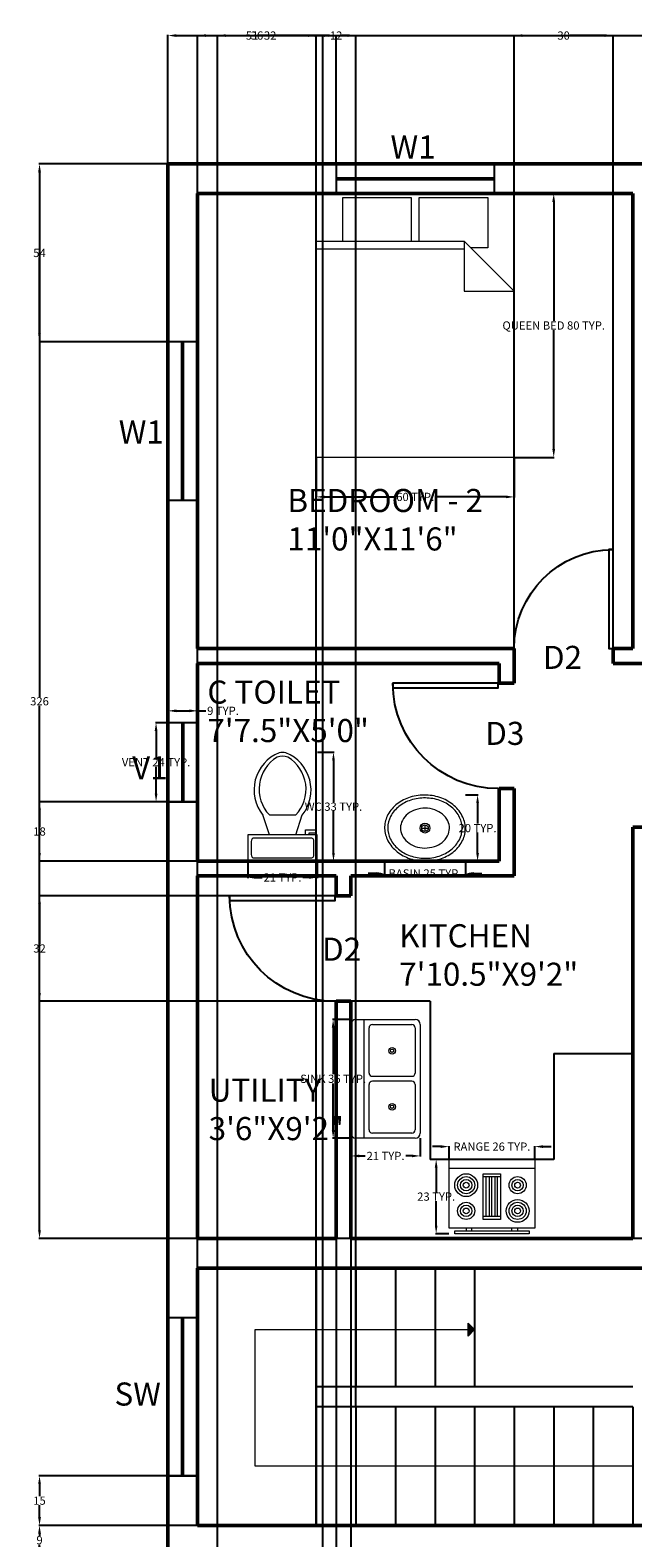
# Model space of a CAD drawing. Units: inches. Extents: x 227 to 711, y 218 to 1048.
# Tile 4 of 5: x 227 to 410, y 590 to 1048. Entities that reach past the tile are written whole.
import ezdxf

# ---------------------------------------------------------------- set-up
doc = ezdxf.new("R2010")
doc.units = ezdxf.units.IN
doc.header["$MEASUREMENT"] = 0
for name, color, linetype, lineweight in [('A-ANNO-DIMS', 2, 'Continuous', 18), ('A-ANNO-SYMB', 85, 'Continuous', 18), ('A-ANNO-TEXT', 70, 'Continuous', 18), ('A-AREA-IDEN', 70, 'Continuous', 25), ('A-FLOR-CASE', 32, 'Continuous', 25), ('A-FLOR-FIXT', 140, 'Continuous', 18), ('A-FURN', 8, 'Continuous', 18), ('A-WALL', 10, 'Continuous', 50), ('DOORS', 30, 'Continuous', 25), ('EQUIPMENTS', 140, 'Continuous', 18), ('STAIRCASE', 220, 'Continuous', 25), ('WINDOWS', 50, 'Continuous', 25)]:
    doc.layers.add(name, color=color, linetype=linetype, lineweight=lineweight)
doc.styles.get("Standard").update_dxf_attribs({"font": 'arial.ttf'})
doc.dimstyles.get("Standard").update_dxf_attribs({"dimtxt": 2.5, "dimasz": 2.5, "dimexe": 0.18, "dimexo": 0.0625, "dimgap": 0.09, "dimtad": 0, "dimtih": 1, "dimtoh": 1, "dimzin": 0, "dimdsep": 46, "dimlunit": 3, "dimtxsty": 'Standard', "dimcen": 0.09, "dimadec": 0, "dimazin": 0, "dimtfac": 1, "dimtofl": 0, "dimtmove": 0, "dimatfit": 3, "dimfxl": 1, "dimtolj": 1, "dimtzin": 0, "dimarcsym": 0})

# ---------------------------------------------------------------- blocks, each defined once
blk = doc.blocks.new('*U2')
for p, q in [((0, 0), (0, -6)), ((40, 0), (40, -6))]:
    blk.add_line(p, q)
blk.add_lwpolyline([(0, 0), (0, 40), (1.75, 40), (1.75, 0)], close=True)
blk.add_arc((0, 0), 40, 0, 90)
blk = doc.blocks.new('Bed - Queen')
for p, q in [((0, -80.00003), (0, 0)), ((0, 0), (59.99999, 0)), ((59.99999, 0), (59.99999, -80.00003)), ((7.99999, -1.2), (28.79998, -1.2)), ((7.99999, -14.4), (7.99999, -1.2)), ((28.79998, -1.2), (28.79998, -14.4)), ((31.19999, -1.2), (51.99999, -1.2)), ((31.19999, -14.4), (31.19999, -1.2)), ((51.99999, -1.2), (51.99999, -16.4)), ((0, -14.4), (44.8, -14.4)), ((44.8, -16.8), (0, -16.8)), ((59.99999, -29.6), (44.8, -14.4)), ((44.8, -14.4), (44.8, -29.6)), ((51.99999, -16.4), (46.79936, -16.4)), ((44.8, -29.6), (59.99999, -29.6)), ((59.99999, -80.00003), (0, -80.00003))]:
    blk.add_line(p, q)
blk = doc.blocks.new('Toilet - top')
for p, q in [((9.5, -6), (9.5, -2)), ((-10, -8.5), (-8, -8.5)), ((-10, -9.5), (-10, -8.5)), ((-8, -8.5), (-8, -8)), ((-7, -8), (-7, -9.5)), ((-4, -8), (-6, -14)), ((4, -8), (6, -14)), ((-7, -9.5), (-10, -9.5)), ((4, -14), (-4, -14))]:
    blk.add_line(p, q)
blk.add_lwpolyline([(10.5, -8), (10.5, 0), (-10.5, 0), (-10.5, -8)], close=True)
for points in [[(-9.5, -2), (-9.5, -6)], [(8.5, -1), (-8.5, -1)], [(-8.5, -7), (8.5, -7)]]:
    blk.add_lwpolyline(points)
for centre, radius, start, end in [((-8.62, -1.88), 0.884, 81.8699, 188.1301), ((8.62, -1.88), 0.884, 351.8699, 98.1301), ((-8.62, -6.12), 0.884, 171.8699, 278.1301), ((8.62, -6.12), 0.884, 261.8699, 8.1301), ((3.52, -21.58), 12.17, 141.4691, 247.9714), ((4.2, -21.82), 11.33, 136.3677, 238.9468), ((-3.52, -21.58), 12.17, 292.0284, 38.5307), ((-4.2, -21.82), 11.33, 301.053, 43.6321), ((0, -27.88), 4, 245.7318, 294.2682), ((0, -29), 4, 254.8605, 285.1395)]:
    blk.add_arc(centre, radius, start, end)
blk = doc.blocks.new('Sink - Oval top')
for p, q in [((-1, 0), (1, 0)), ((0, 1), (0, -1))]:
    blk.add_line(p, q)
for points in [[(-12.23, 0.39, 0.117634), (-11.46, -3.36, 0.104469), (-8.88, -6.8, 0.090016), (-5.08, -9.07, 0.08192), (-0.32, -10.02, 0.08192), (4.49, -9.38, 0.090016), (8.42, -7.36, 0.104469), (11.22, -4.09, 0.117634), (12.23, -0.39, 0.117634), (11.46, 3.36, 0.104469), (8.88, 6.8, 0.090016), (5.08, 9.07, 0.08192), (0.32, 10.02, 0.08192), (-4.49, 9.38, 0.090016), (-8.42, 7.36, 0.104469), (-11.22, 4.09, 0.117634)], [(-11.29, 0.16, 0.118622), (-10.52, -3.25, 0.104678), (-8.07, -6.36, 0.089562), (-4.54, -8.37, 0.081185), (-0.13, -9.15, 0.081185), (4.3, -8.49, 0.089562), (7.89, -6.58, 0.104678), (10.42, -3.55, 0.118622), (11.29, -0.16, 0.118622), (10.52, 3.25, 0.104678), (8.07, 6.36, 0.089562), (4.54, 8.37, 0.081185), (0.13, 9.15, 0.081185), (-4.3, 8.49, 0.089562), (-7.89, 6.58, 0.104678), (-10.42, 3.55, 0.118622)], [(-7.42, 0.08, 0.118283), (-6.91, -2.17, 0.104607), (-5.29, -4.21, 0.089718), (-2.97, -5.53, 0.081436), (-0.07, -6.04, 0.081436), (2.84, -5.59, 0.089718), (5.2, -4.33, 0.104607), (6.86, -2.32, 0.118283), (7.42, -0.08, 0.118283), (6.91, 2.17, 0.104607), (5.29, 4.21, 0.089718), (2.97, 5.53, 0.081436), (0.07, 6.04, 0.081436), (-2.84, 5.59, 0.089718), (-5.2, 4.33, 0.104607), (-6.86, 2.32, 0.118283)]]:
    blk.add_lwpolyline(points, format="xyb", close=True)
for radius in [1.5, 1]:
    blk.add_circle((0, 0), radius)
blk = doc.blocks.new('Range-Oven - 30 in top')
for p, q in [((0, -3), (30, -3)), ((12, -6), (18, -6)), ((13, -20), (13, -6)), ((14, -6), (14, -20)), ((15, -20), (15, -6)), ((16, -6), (16, -20)), ((17, -20), (17, -6)), ((18, -20), (12, -20)), ((6, -24), (6, -25)), ((8, -25), (8, -24)), ((22, -25), (22, -24)), ((24, -24), (24, -25))]:
    blk.add_line(p, q)
for points in [[(0, -24), (0, 0), (30, 0), (30, -24)], [(12, -21), (12, -5), (18, -5), (18, -21)], [(2, -26), (2, -25), (28, -25), (28, -26)]]:
    blk.add_lwpolyline(points, close=True)
for centre, radius in [((6, -9), 4), ((6, -9), 3), ((6, -9), 2), ((6, -9), 1), ((24, -9), 3), ((24, -9), 2), ((24, -9), 1), ((6, -18), 3), ((24, -18), 4), ((24, -18), 3), ((6, -18), 2), ((6, -18), 1), ((24, -18), 2), ((24, -18), 1)]:
    blk.add_circle(centre, radius)
blk = doc.blocks.new('Sink-double - 36 in top')
for p, q in [((-18, -4), (18, -4)), ((-0.75, -18.5), (-0.75, -6.5)), ((0.75, -6.5), (0.75, -18.5))]:
    blk.add_line(p, q)
for points in [[(-16.5, 0), (16.5, 0)], [(-18, -19.5), (-18, -1.5)], [(18, -1.5), (18, -19.5)], [(-16.5, -18.5), (-16.5, -6.5)], [(-15.5, -5.5), (-1.75, -5.5)], [(1.75, -5.5), (15.5, -5.5)], [(16.5, -6.5), (16.5, -18.5)], [(16.5, -21), (-16.5, -21)], [(-1.75, -19.5), (-15.5, -19.5)], [(15.5, -19.5), (1.75, -19.5)]]:
    blk.add_lwpolyline(points)
for centre, radius in [((-8.5, -12.5), 1), ((-8.5, -12.5), 0.5), ((8.5, -12.5), 1), ((8.5, -12.5), 0.5)]:
    blk.add_circle(centre, radius)
for centre, radius, start, end in [((-16.5, -1.5), 1.5, 90, 180), ((16.5, -1.5), 1.5, 0, 90), ((-15.5, -6.5), 1, 90, 180), ((-1.75, -6.5), 1, 0, 90), ((1.75, -6.5), 1, 90, 180), ((15.5, -6.5), 1, 0, 90), ((-16.5, -19.5), 1.5, 180, 270), ((-15.5, -18.5), 1, 180, 270), ((-1.75, -18.5), 1, 270, 0), ((1.75, -18.5), 1, 180, 270), ((15.5, -18.5), 1, 270, 0), ((16.5, -19.5), 1.5, 270, 0)]:
    blk.add_arc(centre, radius, start, end)
blk = doc.blocks.new('WIN-48IN')
for p, q in [((0, 4.75), (48, 4.75)), ((0, 4.25), (48, 4.25))]:
    blk.add_line(p, q)
blk.add_lwpolyline([(0, 0), (48, 0), (48, 9), (0, 9)], close=True)
blk = doc.blocks.new('VENT-V1-24IN')
for p, q in [((4.25, 24), (4.25, 0)), ((4.75, 24), (4.75, 0))]:
    blk.add_line(p, q)
blk.add_lwpolyline([(0, 24), (0, 0), (9, 0), (9, 24)], close=True)
blk = doc.blocks.new('*D22')
at = {"layer": 'A-ANNO-DIMS', "color": 0, "lineweight": -2, "transparency": 16777216}
for p, q in [((374.05, 998.07), (386.17, 998.07)), ((385.99, 995.57), (385.99, 959.52)), ((385.99, 920.56), (385.99, 956.61)), ((374.05, 918.06), (386.17, 918.06))]:
    blk.add_line(p, q, dxfattribs=at)
at = {"layer": 'A-ANNO-DIMS', "color": 0, "transparency": 16777216}
for points in [[(385.57, 995.57), (386.41, 995.57), (385.99, 998.07)], [(385.57, 920.56), (386.41, 920.56), (385.99, 918.06)]]:
    blk.add_solid(points, dxfattribs=at)
at = {"layer": 'Defpoints', "color": 0, "transparency": 16777216}
for p in [(373.99, 998.07), (385.99, 998.07), (373.99, 918.06)]:
    blk.add_point(p, dxfattribs=at)
at = {"layer": 'A-ANNO-DIMS', "color": 0, "transparency": 16777216, "insert": (385.99, 958.06), "char_height": 2.5, "attachment_point": 5}
blk.add_mtext('\\A1;QUEEN BED 80 TYP.', dxfattribs=at)
blk = doc.blocks.new('*D23')
at = {"layer": 'A-ANNO-DIMS', "color": 0, "lineweight": -2, "transparency": 16777216}
for p, q in [((313.99, 918), (313.99, 905.88)), ((373.99, 918), (373.99, 905.88)), ((316.49, 906.06), (337.81, 906.06)), ((371.49, 906.06), (350.17, 906.06))]:
    blk.add_line(p, q, dxfattribs=at)
at = {"layer": 'A-ANNO-DIMS', "color": 0, "transparency": 16777216}
for points in [[(316.49, 906.48), (316.49, 905.65), (313.99, 906.06)], [(371.49, 906.48), (371.49, 905.65), (373.99, 906.06)]]:
    blk.add_solid(points, dxfattribs=at)
at = {"layer": 'Defpoints', "color": 0, "transparency": 16777216}
for p in [(313.99, 918.06), (373.99, 918.06), (373.99, 906.06)]:
    blk.add_point(p, dxfattribs=at)
at = {"layer": 'A-ANNO-DIMS', "color": 0, "transparency": 16777216, "insert": (343.99, 906.06), "char_height": 2.5, "attachment_point": 5}
blk.add_mtext('\\A1;60 TYP.', dxfattribs=at)
blk = doc.blocks.new('*D24')
at = {"layer": 'A-ANNO-DIMS', "color": 0, "lineweight": -2, "transparency": 16777216}
for p, q in [((314.31, 828.61), (319.38, 828.61)), ((319.2, 826.11), (319.2, 813.47)), ((319.2, 798.07), (319.2, 810.7)), ((314.31, 795.57), (319.38, 795.57))]:
    blk.add_line(p, q, dxfattribs=at)
at = {"layer": 'A-ANNO-DIMS', "color": 0, "transparency": 16777216}
for points in [[(318.78, 826.11), (319.62, 826.11), (319.2, 828.61)], [(318.78, 798.07), (319.62, 798.07), (319.2, 795.57)]]:
    blk.add_solid(points, dxfattribs=at)
at = {"layer": 'Defpoints', "color": 0, "transparency": 16777216}
for p in [(314.24, 828.61), (314.24, 795.57), (319.2, 795.57)]:
    blk.add_point(p, dxfattribs=at)
at = {"layer": 'A-ANNO-DIMS', "color": 0, "transparency": 16777216, "insert": (319.2, 812.09), "char_height": 2.5, "attachment_point": 5}
blk.add_mtext('\\A1;WC 33 TYP.', dxfattribs=at)
blk = doc.blocks.new('*D25')
at = {"layer": 'A-ANNO-DIMS', "color": 0, "lineweight": -2, "transparency": 16777216}
for p, q in [((293.24, 795.5), (293.24, 790.43)), ((314.24, 795.5), (314.24, 790.43)), ((295.74, 790.61), (297.55, 790.61)), ((311.74, 790.61), (309.94, 790.61))]:
    blk.add_line(p, q, dxfattribs=at)
at = {"layer": 'A-ANNO-DIMS', "color": 0, "transparency": 16777216}
for points in [[(295.74, 791.02), (295.74, 790.19), (293.24, 790.61)], [(311.74, 791.02), (311.74, 790.19), (314.24, 790.61)]]:
    blk.add_solid(points, dxfattribs=at)
at = {"layer": 'Defpoints', "color": 0, "transparency": 16777216}
for p in [(293.24, 795.57), (314.24, 795.57), (293.24, 790.61)]:
    blk.add_point(p, dxfattribs=at)
at = {"layer": 'A-ANNO-DIMS', "color": 0, "transparency": 16777216, "insert": (303.74, 790.61), "char_height": 2.5, "attachment_point": 5}
blk.add_mtext('\\A1;21 TYP.', dxfattribs=at)
blk = doc.blocks.new('*D26')
at = {"layer": 'A-ANNO-DIMS', "color": 0, "lineweight": -2, "transparency": 16777216}
for p, q in [((332.17, 791.84), (329.67, 791.84)), ((334.67, 795.46), (334.67, 791.66)), ((359.22, 795.46), (359.22, 791.66)), ((361.72, 791.84), (364.22, 791.84))]:
    blk.add_line(p, q, dxfattribs=at)
at = {"layer": 'A-ANNO-DIMS', "color": 0, "transparency": 16777216}
for points in [[(332.17, 792.25), (332.17, 791.42), (334.67, 791.84)], [(361.72, 792.25), (361.72, 791.42), (359.22, 791.84)]]:
    blk.add_solid(points, dxfattribs=at)
at = {"layer": 'Defpoints', "color": 0, "transparency": 16777216}
for p in [(334.67, 795.52), (359.22, 795.52), (359.22, 791.84)]:
    blk.add_point(p, dxfattribs=at)
at = {"layer": 'A-ANNO-DIMS', "color": 0, "transparency": 16777216, "insert": (346.95, 791.84), "char_height": 2.5, "attachment_point": 5}
blk.add_mtext('\\A1;BASIN 25 TYP.', dxfattribs=at)
blk = doc.blocks.new('*D27')
at = {"layer": 'A-ANNO-DIMS', "color": 0, "lineweight": -2, "transparency": 16777216}
for p, q in [((359.28, 815.66), (363.08, 815.66)), ((362.9, 813.16), (362.9, 806.96)), ((362.9, 798.02), (362.9, 804.22)), ((359.28, 795.52), (363.08, 795.52))]:
    blk.add_line(p, q, dxfattribs=at)
at = {"layer": 'A-ANNO-DIMS', "color": 0, "transparency": 16777216}
for points in [[(362.49, 813.16), (363.32, 813.16), (362.9, 815.66)], [(362.49, 798.02), (363.32, 798.02), (362.9, 795.52)]]:
    blk.add_solid(points, dxfattribs=at)
at = {"layer": 'Defpoints', "color": 0, "transparency": 16777216}
for p in [(359.22, 815.66), (362.9, 815.66), (359.22, 795.52)]:
    blk.add_point(p, dxfattribs=at)
at = {"layer": 'A-ANNO-DIMS', "color": 0, "transparency": 16777216, "insert": (362.9, 805.59), "char_height": 2.5, "attachment_point": 5}
blk.add_mtext('\\A1;20 TYP.', dxfattribs=at)
blk = doc.blocks.new('*D28')
at = {"layer": 'A-ANNO-DIMS', "color": 0, "lineweight": -2, "transparency": 16777216}
for p, q in [((268.93, 837.57), (265.21, 837.57)), ((265.39, 835.07), (265.39, 826.91)), ((265.39, 816.07), (265.39, 824.22)), ((268.93, 813.57), (265.21, 813.57))]:
    blk.add_line(p, q, dxfattribs=at)
at = {"layer": 'A-ANNO-DIMS', "color": 0, "transparency": 16777216}
for points in [[(264.97, 835.07), (265.81, 835.07), (265.39, 837.57)], [(264.97, 816.07), (265.81, 816.07), (265.39, 813.57)]]:
    blk.add_solid(points, dxfattribs=at)
at = {"layer": 'Defpoints', "color": 0, "transparency": 16777216}
for p in [(265.39, 837.57), (268.99, 837.57), (268.99, 813.57)]:
    blk.add_point(p, dxfattribs=at)
at = {"layer": 'A-ANNO-DIMS', "color": 0, "transparency": 16777216, "insert": (265.39, 825.57), "char_height": 2.5, "attachment_point": 5}
blk.add_mtext('\\A1;VENT 24 TYP.', dxfattribs=at)
blk = doc.blocks.new('*D29')
at = {"layer": 'A-ANNO-DIMS', "color": 0, "lineweight": -2, "transparency": 16777216}
for p, q in [((268.99, 837.63), (268.99, 841.35)), ((271.49, 841.17), (275.49, 841.17)), ((277.99, 837.63), (277.99, 841.35)), ((277.99, 841.17), (280.49, 841.17))]:
    blk.add_line(p, q, dxfattribs=at)
at = {"layer": 'A-ANNO-DIMS', "color": 0, "transparency": 16777216}
for points in [[(271.49, 841.58), (271.49, 840.75), (268.99, 841.17)], [(275.49, 841.58), (275.49, 840.75), (277.99, 841.17)]]:
    blk.add_solid(points, dxfattribs=at)
at = {"layer": 'Defpoints', "color": 0, "transparency": 16777216}
for p in [(268.99, 837.57), (277.99, 841.17), (277.99, 837.57)]:
    blk.add_point(p, dxfattribs=at)
at = {"layer": 'A-ANNO-DIMS', "color": 0, "transparency": 16777216, "insert": (285.69, 841.17), "char_height": 2.5, "attachment_point": 5}
blk.add_mtext('\\A1;9 TYP.', dxfattribs=at)
blk = doc.blocks.new('*D30')
at = {"layer": 'A-ANNO-DIMS', "color": 0, "lineweight": -2, "transparency": 16777216}
for p, q in [((351.74, 708.97), (349.24, 708.97)), ((354.24, 705.13), (354.24, 709.15)), ((380.24, 705.13), (380.24, 709.15)), ((382.74, 708.97), (385.24, 708.97))]:
    blk.add_line(p, q, dxfattribs=at)
at = {"layer": 'A-ANNO-DIMS', "color": 0, "transparency": 16777216}
for points in [[(351.74, 709.38), (351.74, 708.55), (354.24, 708.97)], [(382.74, 709.38), (382.74, 708.55), (380.24, 708.97)]]:
    blk.add_solid(points, dxfattribs=at)
at = {"layer": 'Defpoints', "color": 0, "transparency": 16777216}
for p in [(380.24, 708.97), (354.24, 705.07), (380.24, 705.07)]:
    blk.add_point(p, dxfattribs=at)
at = {"layer": 'A-ANNO-DIMS', "color": 0, "transparency": 16777216, "insert": (367.24, 708.97), "char_height": 2.5, "attachment_point": 5}
blk.add_mtext('\\A1;RANGE 26 TYP.', dxfattribs=at)
blk = doc.blocks.new('*D31')
at = {"layer": 'A-ANNO-DIMS', "color": 0, "lineweight": -2, "transparency": 16777216}
for p, q in [((354.18, 705.07), (350.16, 705.07)), ((350.34, 702.57), (350.34, 695.17)), ((350.34, 685.03), (350.34, 692.43)), ((354.18, 682.53), (350.16, 682.53))]:
    blk.add_line(p, q, dxfattribs=at)
at = {"layer": 'A-ANNO-DIMS', "color": 0, "transparency": 16777216}
for points in [[(349.92, 702.57), (350.76, 702.57), (350.34, 705.07)], [(349.92, 685.03), (350.76, 685.03), (350.34, 682.53)]]:
    blk.add_solid(points, dxfattribs=at)
at = {"layer": 'Defpoints', "color": 0, "transparency": 16777216}
for p in [(350.34, 705.07), (354.24, 705.07), (354.24, 682.53)]:
    blk.add_point(p, dxfattribs=at)
at = {"layer": 'A-ANNO-DIMS', "color": 0, "transparency": 16777216, "insert": (350.34, 693.8), "char_height": 2.5, "attachment_point": 5}
blk.add_mtext('\\A1;23 TYP.', dxfattribs=at)
blk = doc.blocks.new('*D32')
at = {"layer": 'A-ANNO-DIMS', "color": 0, "lineweight": -2, "transparency": 16777216}
for p, q in [((324.43, 747.54), (318.91, 747.54)), ((319.09, 745.04), (319.09, 730.92)), ((319.09, 714.04), (319.09, 728.15)), ((324.43, 711.54), (318.91, 711.54))]:
    blk.add_line(p, q, dxfattribs=at)
at = {"layer": 'A-ANNO-DIMS', "color": 0, "transparency": 16777216}
for points in [[(318.67, 745.04), (319.51, 745.04), (319.09, 747.54)], [(318.67, 714.04), (319.51, 714.04), (319.09, 711.54)]]:
    blk.add_solid(points, dxfattribs=at)
at = {"layer": 'Defpoints', "color": 0, "transparency": 16777216}
for p in [(319.09, 747.54), (324.49, 747.54), (324.49, 711.54)]:
    blk.add_point(p, dxfattribs=at)
at = {"layer": 'A-ANNO-DIMS', "color": 0, "transparency": 16777216, "insert": (319.09, 729.54), "char_height": 2.5, "attachment_point": 5}
blk.add_mtext('\\A1;SINK 36 TYP.', dxfattribs=at)
blk = doc.blocks.new('*D33')
at = {"layer": 'A-ANNO-DIMS', "color": 0, "lineweight": -2, "transparency": 16777216}
for p, q in [((324.49, 711.48), (324.49, 705.96)), ((345.49, 711.48), (345.49, 705.96)), ((326.99, 706.14), (328.79, 706.14)), ((342.99, 706.14), (341.19, 706.14))]:
    blk.add_line(p, q, dxfattribs=at)
at = {"layer": 'A-ANNO-DIMS', "color": 0, "transparency": 16777216}
for points in [[(326.99, 706.55), (326.99, 705.72), (324.49, 706.14)], [(342.99, 706.55), (342.99, 705.72), (345.49, 706.14)]]:
    blk.add_solid(points, dxfattribs=at)
at = {"layer": 'Defpoints', "color": 0, "transparency": 16777216}
for p in [(324.49, 711.54), (345.49, 711.54), (324.49, 706.14)]:
    blk.add_point(p, dxfattribs=at)
at = {"layer": 'A-ANNO-DIMS', "color": 0, "transparency": 16777216, "insert": (334.99, 706.14), "char_height": 2.5, "attachment_point": 5}
blk.add_mtext('\\A1;21 TYP.', dxfattribs=at)
blk = doc.blocks.new('*D44')
at = {"layer": 'A-ANNO-DIMS', "color": 0, "lineweight": -2, "transparency": 16777216}
for p, q in [((268.99, 1007.13), (268.99, 1046.2)), ((271.49, 1046.02), (464.87, 1046.02)), ((666.99, 1046.02), (473.61, 1046.02)), ((669.49, 1007.13), (669.49, 1046.2))]:
    blk.add_line(p, q, dxfattribs=at)
at = {"layer": 'A-ANNO-DIMS', "color": 0, "transparency": 16777216}
for points in [[(271.49, 1046.43), (271.49, 1045.6), (268.99, 1046.02)], [(666.99, 1046.43), (666.99, 1045.6), (669.49, 1046.02)]]:
    blk.add_solid(points, dxfattribs=at)
at = {"layer": 'Defpoints', "color": 0, "transparency": 16777216}
for p in [(669.49, 1046.02), (268.99, 1007.07), (669.49, 1007.07)]:
    blk.add_point(p, dxfattribs=at)
at = {"layer": 'A-ANNO-DIMS', "color": 0, "transparency": 16777216, "insert": (469.24, 1046.02), "char_height": 2.5, "attachment_point": 5}
blk.add_mtext('\\A1;400.5', dxfattribs=at)
blk = doc.blocks.new('*D51')
at = {"layer": 'A-ANNO-DIMS', "color": 0, "lineweight": -2, "transparency": 16777216}
for p, q in [((268.93, 1007.07), (229.86, 1007.07)), ((230.04, 1004.57), (230.04, 845.43)), ((230.04, 683.57), (230.04, 842.7)), ((459.43, 681.07), (229.86, 681.07))]:
    blk.add_line(p, q, dxfattribs=at)
at = {"layer": 'A-ANNO-DIMS', "color": 0, "transparency": 16777216}
for points in [[(229.62, 1004.57), (230.46, 1004.57), (230.04, 1007.07)], [(229.62, 683.57), (230.46, 683.57), (230.04, 681.07)]]:
    blk.add_solid(points, dxfattribs=at)
at = {"layer": 'Defpoints', "color": 0, "transparency": 16777216}
for p in [(230.04, 1007.07), (268.99, 1007.07), (459.49, 681.07)]:
    blk.add_point(p, dxfattribs=at)
at = {"layer": 'A-ANNO-DIMS', "color": 0, "transparency": 16777216, "insert": (230.04, 844.07), "char_height": 2.5, "attachment_point": 5}
blk.add_mtext('\\A1;326', dxfattribs=at)
blk = doc.blocks.new('*D52')
at = {"layer": 'A-ANNO-DIMS', "color": 0, "lineweight": -2, "transparency": 16777216}
for p, q in [((277.93, 594.07), (229.86, 594.07)), ((230.04, 591.57), (230.04, 590.93)), ((230.04, 587.57), (230.04, 588.2)), ((277.93, 585.07), (229.86, 585.07))]:
    blk.add_line(p, q, dxfattribs=at)
at = {"layer": 'A-ANNO-DIMS', "color": 0, "transparency": 16777216}
for points in [[(229.62, 591.57), (230.46, 591.57), (230.04, 594.07)], [(229.62, 587.57), (230.46, 587.57), (230.04, 585.07)]]:
    blk.add_solid(points, dxfattribs=at)
at = {"layer": 'Defpoints', "color": 0, "transparency": 16777216}
for p in [(230.04, 594.07), (277.99, 594.07), (277.99, 585.07)]:
    blk.add_point(p, dxfattribs=at)
at = {"layer": 'A-ANNO-DIMS', "color": 0, "transparency": 16777216, "insert": (230.04, 589.57), "char_height": 2.5, "attachment_point": 5}
blk.add_mtext('\\A1;9', dxfattribs=at)
blk = doc.blocks.new('*D54')
at = {"layer": 'A-ANNO-DIMS', "color": 0, "lineweight": -2, "transparency": 16777216}
for p, q in [((373.99, 860.13), (373.99, 1046.2)), ((376.49, 1046.02), (387.11, 1046.02)), ((401.49, 1046.02), (390.87, 1046.02)), ((403.99, 860.13), (403.99, 1046.2))]:
    blk.add_line(p, q, dxfattribs=at)
at = {"layer": 'A-ANNO-DIMS', "color": 0, "transparency": 16777216}
for points in [[(376.49, 1046.43), (376.49, 1045.6), (373.99, 1046.02)], [(401.49, 1046.43), (401.49, 1045.6), (403.99, 1046.02)]]:
    blk.add_solid(points, dxfattribs=at)
at = {"layer": 'Defpoints', "color": 0, "transparency": 16777216}
for p in [(403.99, 1046.02), (373.99, 860.07), (403.99, 860.07)]:
    blk.add_point(p, dxfattribs=at)
at = {"layer": 'A-ANNO-DIMS', "color": 0, "transparency": 16777216, "insert": (388.99, 1046.02), "char_height": 2.5, "attachment_point": 5}
blk.add_mtext('\\A1;30', dxfattribs=at)
blk = doc.blocks.new('*D55')
at = {"layer": 'A-ANNO-DIMS', "color": 0, "lineweight": -2, "transparency": 16777216}
for p, q in [((283.99, 451.13), (283.99, 1046.2)), ((286.49, 1046.02), (298.12, 1046.02)), ((313.49, 1046.02), (301.86, 1046.02)), ((315.99, 451.13), (315.99, 1046.2))]:
    blk.add_line(p, q, dxfattribs=at)
at = {"layer": 'A-ANNO-DIMS', "color": 0, "transparency": 16777216}
for points in [[(286.49, 1046.43), (286.49, 1045.6), (283.99, 1046.02)], [(313.49, 1046.43), (313.49, 1045.6), (315.99, 1046.02)]]:
    blk.add_solid(points, dxfattribs=at)
at = {"layer": 'Defpoints', "color": 0, "transparency": 16777216}
for p in [(315.99, 1046.02), (283.99, 451.07), (315.99, 451.07)]:
    blk.add_point(p, dxfattribs=at)
at = {"layer": 'A-ANNO-DIMS', "color": 0, "transparency": 16777216, "insert": (299.99, 1046.02), "char_height": 2.5, "attachment_point": 5}
blk.add_mtext('\\A1;32', dxfattribs=at)
blk = doc.blocks.new('*D57')
at = {"layer": 'A-ANNO-DIMS', "color": 0, "lineweight": -2, "transparency": 16777216}
for p, q in [((277.99, 594.13), (277.99, 1046.2)), ((280.49, 1046.02), (294.11, 1046.02)), ((311.49, 1046.02), (297.87, 1046.02)), ((313.99, 594.13), (313.99, 1046.2))]:
    blk.add_line(p, q, dxfattribs=at)
at = {"layer": 'A-ANNO-DIMS', "color": 0, "transparency": 16777216}
for points in [[(280.49, 1046.43), (280.49, 1045.6), (277.99, 1046.02)], [(311.49, 1046.43), (311.49, 1045.6), (313.99, 1046.02)]]:
    blk.add_solid(points, dxfattribs=at)
at = {"layer": 'Defpoints', "color": 0, "transparency": 16777216}
for p in [(313.99, 1046.02), (277.99, 594.07), (313.99, 594.07)]:
    blk.add_point(p, dxfattribs=at)
at = {"layer": 'A-ANNO-DIMS', "color": 0, "transparency": 16777216, "insert": (295.99, 1046.02), "char_height": 2.5, "attachment_point": 5}
blk.add_mtext('\\A1;36', dxfattribs=at)
blk = doc.blocks.new('*D58')
at = {"layer": 'A-ANNO-DIMS', "color": 0, "lineweight": -2, "transparency": 16777216}
for p, q in [((313.99, 630.13), (313.99, 1046.2)), ((316.49, 1046.02), (318.24, 1046.02)), ((323.49, 1046.02), (321.74, 1046.02)), ((325.99, 630.13), (325.99, 1046.2))]:
    blk.add_line(p, q, dxfattribs=at)
at = {"layer": 'A-ANNO-DIMS', "color": 0, "transparency": 16777216}
for points in [[(316.49, 1046.43), (316.49, 1045.6), (313.99, 1046.02)], [(323.49, 1046.43), (323.49, 1045.6), (325.99, 1046.02)]]:
    blk.add_solid(points, dxfattribs=at)
at = {"layer": 'Defpoints', "color": 0, "transparency": 16777216}
for p in [(325.99, 1046.02), (313.99, 630.07), (325.99, 630.07)]:
    blk.add_point(p, dxfattribs=at)
at = {"layer": 'A-ANNO-DIMS', "color": 0, "transparency": 16777216, "insert": (319.99, 1046.02), "char_height": 2.5, "attachment_point": 5}
blk.add_mtext('\\A1;12', dxfattribs=at)
blk = doc.blocks.new('*D61')
at = {"layer": 'A-ANNO-DIMS', "color": 0, "lineweight": -2, "transparency": 16777216}
for p, q in [((268.99, 1007.13), (268.99, 1046.2)), ((271.49, 1046.02), (292.85, 1046.02)), ((317.49, 1046.02), (296.13, 1046.02)), ((319.99, 1007.13), (319.99, 1046.2))]:
    blk.add_line(p, q, dxfattribs=at)
at = {"layer": 'A-ANNO-DIMS', "color": 0, "transparency": 16777216}
for points in [[(271.49, 1046.43), (271.49, 1045.6), (268.99, 1046.02)], [(317.49, 1046.43), (317.49, 1045.6), (319.99, 1046.02)]]:
    blk.add_solid(points, dxfattribs=at)
at = {"layer": 'Defpoints', "color": 0, "transparency": 16777216}
for p in [(319.99, 1046.02), (268.99, 1007.07), (319.99, 1007.07)]:
    blk.add_point(p, dxfattribs=at)
at = {"layer": 'A-ANNO-DIMS', "color": 0, "transparency": 16777216, "insert": (294.49, 1046.02), "char_height": 2.5, "attachment_point": 5}
blk.add_mtext('\\A1;51', dxfattribs=at)
blk = doc.blocks.new('*D63')
at = {"layer": 'A-ANNO-DIMS', "color": 0, "lineweight": -2, "transparency": 16777216}
for p, q in [((268.93, 1007.07), (229.86, 1007.07)), ((230.04, 1004.57), (230.04, 981.43)), ((230.04, 955.57), (230.04, 978.7)), ((268.93, 953.07), (229.86, 953.07))]:
    blk.add_line(p, q, dxfattribs=at)
at = {"layer": 'A-ANNO-DIMS', "color": 0, "transparency": 16777216}
for points in [[(229.62, 1004.57), (230.46, 1004.57), (230.04, 1007.07)], [(229.62, 955.57), (230.46, 955.57), (230.04, 953.07)]]:
    blk.add_solid(points, dxfattribs=at)
at = {"layer": 'Defpoints', "color": 0, "transparency": 16777216}
for p in [(230.04, 1007.07), (268.99, 1007.07), (268.99, 953.07)]:
    blk.add_point(p, dxfattribs=at)
at = {"layer": 'A-ANNO-DIMS', "color": 0, "transparency": 16777216, "insert": (230.04, 980.07), "char_height": 2.5, "attachment_point": 5}
blk.add_mtext('\\A1;54', dxfattribs=at)
blk = doc.blocks.new('*D65')
at = {"layer": 'A-ANNO-DIMS', "color": 0, "lineweight": -2, "transparency": 16777216}
for p, q in [((319.99, 681), (319.99, 219.94)), ((324.49, 681), (324.49, 219.94)), ((317.49, 220.12), (314.99, 220.12)), ((326.99, 220.12), (329.49, 220.12))]:
    blk.add_line(p, q, dxfattribs=at)
at = {"layer": 'A-ANNO-DIMS', "color": 0, "transparency": 16777216}
for points in [[(317.49, 220.53), (317.49, 219.7), (319.99, 220.12)], [(326.99, 220.53), (326.99, 219.7), (324.49, 220.12)]]:
    blk.add_solid(points, dxfattribs=at)
at = {"layer": 'Defpoints', "color": 0, "transparency": 16777216}
for p in [(319.99, 681.07), (324.49, 681.07), (324.49, 220.12)]:
    blk.add_point(p, dxfattribs=at)
at = {"layer": 'A-ANNO-DIMS', "color": 0, "transparency": 16777216, "insert": (331.92, 220.12), "char_height": 2.5, "attachment_point": 5}
blk.add_mtext('\\A1;4.5', dxfattribs=at)
blk = doc.blocks.new('*D66')
at = {"layer": 'A-ANNO-DIMS', "color": 0, "lineweight": -2, "transparency": 16777216}
for p, q in [((277.93, 813.57), (229.86, 813.57)), ((230.04, 811.07), (230.04, 805.93)), ((230.04, 798.07), (230.04, 803.2)), ((277.93, 795.57), (229.86, 795.57))]:
    blk.add_line(p, q, dxfattribs=at)
at = {"layer": 'A-ANNO-DIMS', "color": 0, "transparency": 16777216}
for points in [[(229.62, 811.07), (230.46, 811.07), (230.04, 813.57)], [(229.62, 798.07), (230.46, 798.07), (230.04, 795.57)]]:
    blk.add_solid(points, dxfattribs=at)
at = {"layer": 'Defpoints', "color": 0, "transparency": 16777216}
for p in [(230.04, 813.57), (277.99, 813.57), (277.99, 795.57)]:
    blk.add_point(p, dxfattribs=at)
at = {"layer": 'A-ANNO-DIMS', "color": 0, "transparency": 16777216, "insert": (230.04, 804.57), "char_height": 2.5, "attachment_point": 5}
blk.add_mtext('\\A1;18', dxfattribs=at)
blk = doc.blocks.new('*D67')
at = {"layer": 'A-ANNO-DIMS', "color": 0, "lineweight": -2, "transparency": 16777216}
for p, q in [((319.93, 785.07), (229.86, 785.07)), ((230.04, 782.57), (230.04, 770.43)), ((230.04, 755.57), (230.04, 767.7)), ((319.93, 753.07), (229.86, 753.07))]:
    blk.add_line(p, q, dxfattribs=at)
at = {"layer": 'A-ANNO-DIMS', "color": 0, "transparency": 16777216}
for points in [[(229.62, 782.57), (230.46, 782.57), (230.04, 785.07)], [(229.62, 755.57), (230.46, 755.57), (230.04, 753.07)]]:
    blk.add_solid(points, dxfattribs=at)
at = {"layer": 'Defpoints', "color": 0, "transparency": 16777216}
for p in [(230.04, 785.07), (319.99, 785.07), (319.99, 753.07)]:
    blk.add_point(p, dxfattribs=at)
at = {"layer": 'A-ANNO-DIMS', "color": 0, "transparency": 16777216, "insert": (230.04, 769.07), "char_height": 2.5, "attachment_point": 5}
blk.add_mtext('\\A1;32', dxfattribs=at)
blk = doc.blocks.new('*D68')
at = {"layer": 'A-ANNO-DIMS', "color": 0, "lineweight": -2, "transparency": 16777216}
for p, q in [((277.93, 609.07), (229.86, 609.07)), ((230.04, 606.57), (230.04, 602.93)), ((230.04, 596.57), (230.04, 600.2)), ((277.93, 594.07), (229.86, 594.07))]:
    blk.add_line(p, q, dxfattribs=at)
at = {"layer": 'A-ANNO-DIMS', "color": 0, "transparency": 16777216}
for points in [[(229.62, 606.57), (230.46, 606.57), (230.04, 609.07)], [(229.62, 596.57), (230.46, 596.57), (230.04, 594.07)]]:
    blk.add_solid(points, dxfattribs=at)
at = {"layer": 'Defpoints', "color": 0, "transparency": 16777216}
for p in [(230.04, 609.07), (277.99, 609.07), (277.99, 594.07)]:
    blk.add_point(p, dxfattribs=at)
at = {"layer": 'A-ANNO-DIMS', "color": 0, "transparency": 16777216, "insert": (230.04, 601.57), "char_height": 2.5, "attachment_point": 5}
blk.add_mtext('\\A1;15', dxfattribs=at)

msp = doc.modelspace()

# ---------------------------------------------------------------- hatches: boundary and pattern name
at = {"layer": 'A-ANNO-SYMB'}
h = msp.add_hatch(color=256, dxfattribs=at)
h.dxf.hatch_style = 1
h.paths.add_polyline_path([(360.004, 655.449), (360.004, 653.48), (361.99, 653.48)])
h.paths.add_polyline_path([(361.99, 653.48), (360.004, 653.48), (360.004, 651.477)])

# ---------------------------------------------------------------- linework, layer by layer
for p, q in [((360.004, 655.449), (361.99, 653.48)), ((360.004, 651.477), (360.004, 655.449)), ((295.48, 612.065), (295.48, 653.48)), ((295.48, 653.48), (361.99, 653.48)), ((361.99, 653.48), (360.004, 651.477)), ((409.99, 612.065), (295.48, 612.065))]:
    msp.add_line(p, q, dxfattribs=at)
at = {"layer": 'A-FLOR-CASE'}
for p, q in [((348.49, 753.065), (324.49, 753.065)), ((348.49, 753.065), (348.49, 705.065)), ((385.99, 737.196), (385.99, 705.065)), ((385.99, 737.196), (409.99, 737.196)), ((385.99, 705.065), (348.49, 705.065))]:
    msp.add_line(p, q, dxfattribs=at)
at = {"layer": 'A-WALL'}
for p, q in [((277.99, 998.065), (277.99, 860.065)), ((409.99, 998.065), (277.99, 998.065)), ((409.99, 998.065), (409.99, 860.065)), ((373.99, 860.065), (277.99, 860.065)), ((373.99, 860.065), (373.99, 849.565)), ((409.99, 860.065), (403.99, 860.065)), ((403.99, 860.065), (403.99, 855.565)), ((277.99, 855.565), (277.99, 795.565)), ((369.49, 855.565), (277.99, 855.565)), ((369.49, 855.565), (369.49, 849.565)), ((409.99, 855.565), (403.99, 855.565)), ((409.99, 855.565), (414.49, 855.565)), ((369.49, 849.565), (373.99, 849.565)), ((369.49, 817.565), (373.99, 817.565)), ((369.49, 817.565), (369.49, 795.565)), ((373.99, 817.565), (373.99, 791.065)), ((409.99, 805.861), (409.99, 681.065)), ((409.99, 805.861), (414.49, 805.861)), ((369.49, 795.565), (277.99, 795.565)), ((277.99, 791.065), (277.99, 681.065)), ((319.99, 791.065), (277.99, 791.065)), ((319.99, 791.065), (319.99, 785.065)), ((373.99, 791.065), (324.49, 791.065)), ((324.49, 791.065), (324.49, 785.065)), ((319.99, 785.065), (324.49, 785.065)), ((319.99, 753.065), (324.49, 753.065)), ((319.99, 753.065), (319.99, 681.065)), ((324.49, 753.065), (324.49, 681.065)), ((319.99, 681.065), (277.99, 681.065)), ((409.99, 681.065), (324.49, 681.065)), ((414.49, 672.065), (277.99, 672.065)), ((277.99, 672.065), (277.99, 594.065)), ((414.49, 594.065), (277.99, 594.065))]:
    msp.add_line(p, q, dxfattribs=at)
msp.add_lwpolyline([(414.49, 1007.065), (268.99, 1007.065), (268.99, 259.065), (414.49, 259.065)], dxfattribs=at)
at = {"layer": 'STAIRCASE'}
for p, q in [((313.99, 672.065), (313.99, 594.065)), ((325.99, 672.065), (325.99, 636.065)), ((337.99, 672.065), (337.99, 636.065)), ((349.99, 672.065), (349.99, 636.065)), ((361.99, 672.065), (361.99, 636.065)), ((409.99, 636.065), (313.99, 636.065)), ((409.99, 630.065), (313.99, 630.065)), ((325.99, 630.065), (325.99, 594.065)), ((337.99, 630.065), (337.99, 594.065)), ((349.99, 630.065), (349.99, 594.065)), ((361.99, 630.065), (361.99, 594.065)), ((373.99, 630.065), (373.99, 594.065)), ((385.99, 630.065), (385.99, 594.065)), ((397.99, 630.065), (397.99, 594.065)), ((409.99, 630.065), (409.99, 594.065))]:
    msp.add_line(p, q, dxfattribs=at)

# ---------------------------------------------------------------- block references
at = {"layer": 'A-FLOR-FIXT'}
for name, p, rotation in [('Toilet - top', (303.744, 795.565), 180), ('Sink-double - 36 in top', (324.49, 729.538), 90)]:
    msp.add_blockref(name, p, dxfattribs=dict(at, rotation=rotation))
msp.add_blockref('Sink - Oval top', (346.947, 805.589), dxfattribs=at)
at = {"layer": 'A-FURN'}
msp.add_blockref('Bed - Queen', (313.99, 998.065), dxfattribs=at)
at = {"layer": 'DOORS', "xscale": -0.75, "yscale": 0.75, "zscale": 0.75}
msp.add_blockref('*U2', (403.99, 860.065), dxfattribs=at)
at = {"layer": 'DOORS', "xscale": -0.8, "yscale": 0.8, "zscale": 0.8, "rotation": 90}
for p in [(369.19, 849.565), (319.69, 785.065)]:
    msp.add_blockref('*U2', p, dxfattribs=at)
at = {"layer": 'EQUIPMENTS', "xscale": 0.8666665333333337, "yscale": 0.8666665333333337, "zscale": 0.8666665333333337}
msp.add_blockref('Range-Oven - 30 in top', (354.24, 705.065), dxfattribs=at)
at = {"layer": 'WINDOWS'}
for name, p in [('WIN-48IN', (319.99, 998.065)), ('VENT-V1-24IN', (268.99, 813.565))]:
    msp.add_blockref(name, p, dxfattribs=at)
for p, rotation in [((277.99, 905.065), 89.99999999999999), ((277.99, 609.065), 90.00000000000003)]:
    msp.add_blockref('WIN-48IN', p, dxfattribs=dict(at, rotation=rotation))

# ---------------------------------------------------------------- texts
at = {"layer": 'A-ANNO-TEXT', "char_height": 7, "attachment_point": 1}
for s, insert in [('W1', (336.484, 1015.705)), ('W1', (254.067, 929.245)), ('D2', (382.715, 860.879)), ('D3', (365.216, 837.824)), ('V1', (258.113, 827.382)), ('D2', (315.73, 772.346)), ('SW', (252.769, 637.402))]:
    msp.add_mtext_dynamic_manual_height_columns(s, width=74.58955, gutter_width=1, heights=[0], dxfattribs=dict(at, insert=insert))
at = {"layer": 'A-AREA-IDEN', "char_height": 7, "attachment_point": 1}
for s, insert in [('BEDROOM - 2\\P11\'0"X11\'6"', (305.211, 908.477)), ('C TOILET\\P7\'7.5"X5\'0"', (280.946, 850.349)), ('KITCHEN\\P7\'10.5"X9\'2"', (339.125, 776.432)), ('UTILITY\\P3\'6"X9\'2"', (281.342, 729.594))]:
    msp.add_mtext_dynamic_manual_height_columns(s, width=74.58955, gutter_width=1, heights=[0], dxfattribs=dict(at, insert=insert))

# ---------------------------------------------------------------- dimensions: what is measured, and where the dimension line sits
at = {"layer": 'A-ANNO-DIMS'}
for base, p1, p2, override, picture, middle in [((669.49, 1046.015), (268.99, 1007.065), (669.49, 1007.065), {"dimdec": 1, "dimlfac": 1, "dimrnd": 0, "dimzin": 0, "dimdsep": 46, "dimlunit": 2}, '*D44', (469.24, 1046.015)), ((319.99, 1046.015), (268.99, 1007.065), (319.99, 1007.065), {"dimdec": 0, "dimlfac": 1, "dimrnd": 0, "dimzin": 0, "dimdsep": 46, "dimlunit": 2}, '*D61', (294.49, 1046.015)), ((313.99, 1046.015), (277.99, 594.065), (313.99, 594.065), {"dimdec": 0, "dimlfac": 1, "dimrnd": 0, "dimzin": 0, "dimdsep": 46, "dimlunit": 2}, '*D57', (295.99, 1046.015)), ((315.99, 1046.015), (283.99, 451.065), (315.99, 451.065), {"dimdec": 0, "dimlfac": 1, "dimrnd": 0, "dimzin": 0, "dimdsep": 46, "dimlunit": 2}, '*D55', (299.99, 1046.015)), ((325.99, 1046.015), (313.99, 630.065), (325.99, 630.065), {"dimdec": 0, "dimlfac": 1, "dimrnd": 0, "dimzin": 0, "dimdsep": 46, "dimlunit": 2}, '*D58', (319.99, 1046.015)), ((403.99, 1046.015), (373.99, 860.065), (403.99, 860.065), {"dimdec": 0, "dimlfac": 1, "dimrnd": 0, "dimzin": 0, "dimdsep": 46, "dimlunit": 2}, '*D54', (388.99, 1046.015)), ((324.49, 220.115), (319.99, 681.065), (324.49, 681.065), {"dimdec": 1, "dimlfac": 1, "dimrnd": 0, "dimzin": 0, "dimdsep": 46, "dimlunit": 2}, '*D65', (331.915, 220.115))]:
    dim = msp.add_linear_dim(base=base, p1=p1, p2=p2, dimstyle='Standard', override=override, dxfattribs=at)
    dim.commit()
    dim.dimension.update_dxf_attribs({"geometry": picture, "text_midpoint": middle})
for base, p1, p2, picture, middle in [((230.04, 1007.065), (459.49, 681.065), (268.99, 1007.065), '*D51', (230.04, 844.065)), ((230.04, 1007.065), (268.99, 953.065), (268.99, 1007.065), '*D63', (230.04, 980.065)), ((230.04, 813.565), (277.99, 795.565), (277.99, 813.565), '*D66', (230.04, 804.565)), ((230.04, 785.065), (319.99, 753.065), (319.99, 785.065), '*D67', (230.04, 769.065)), ((230.04, 609.065), (277.99, 594.065), (277.99, 609.065), '*D68', (230.04, 601.565)), ((230.04, 594.065), (277.99, 585.065), (277.99, 594.065), '*D52', (230.04, 589.565))]:
    dim = msp.add_linear_dim(base=base, p1=p1, p2=p2, angle=90, dimstyle='Standard', override={"dimdec": 0, "dimlfac": 1, "dimrnd": 0, "dimzin": 0, "dimdsep": 46, "dimlunit": 2}, dxfattribs=at)
    dim.commit()
    dim.dimension.update_dxf_attribs({"geometry": picture, "text_midpoint": middle})
for base, p1, p2, angle, text, picture, middle in [((385.99, 998.065), (373.99, 918.065), (373.99, 998.065), 90, 'QUEEN BED <> TYP.', '*D22', (385.99, 958.065)), ((265.39, 837.565), (268.99, 813.565), (268.99, 837.565), 90, 'VENT <> TYP.', '*D28', (265.39, 825.565)), ((319.201, 795.565), (314.244, 828.611), (314.244, 795.565), 270, 'WC <> TYP.', '*D24', (319.201, 812.088)), ((362.905, 815.657), (359.222, 795.52), (359.222, 815.657), 90, '<> TYP.', '*D27', (362.905, 805.589)), ((293.244, 790.608), (314.244, 795.565), (293.244, 795.565), 180, '<> TYP.', '*D25', (303.744, 790.608)), ((319.09, 747.538), (324.49, 711.538), (324.49, 747.538), 90, 'SINK <> TYP.', '*D32', (319.09, 729.538)), ((324.49, 706.138), (345.49, 711.538), (324.49, 711.538), 180, '<> TYP.', '*D33', (334.99, 706.138)), ((350.34, 705.065), (354.24, 682.532), (354.24, 705.065), 90, '<> TYP.', '*D31', (350.34, 693.798))]:
    dim = msp.add_linear_dim(base=base, p1=p1, p2=p2, angle=angle, text=text, dimstyle='Standard', override={"dimdec": 0, "dimlfac": 1, "dimrnd": 0, "dimzin": 0, "dimdsep": 46, "dimlunit": 2}, dxfattribs=at)
    dim.commit()
    dim.dimension.update_dxf_attribs({"geometry": picture, "text_midpoint": middle})
for base, p1, p2, text, picture, middle in [((373.99, 906.065), (313.99, 918.065), (373.99, 918.065), '<> TYP.', '*D23', (343.99, 906.065)), ((277.99, 841.165), (268.99, 837.565), (277.99, 837.565), '<> TYP.', '*D29', (285.693, 841.165)), ((359.222, 791.838), (334.671, 795.52), (359.222, 795.52), 'BASIN <> TYP.', '*D26', (346.947, 791.838)), ((380.24, 708.965), (354.24, 705.065), (380.24, 705.065), 'RANGE <> TYP.', '*D30', (367.24, 708.965))]:
    dim = msp.add_linear_dim(base=base, p1=p1, p2=p2, text=text, dimstyle='Standard', override={"dimdec": 0, "dimlfac": 1, "dimrnd": 0, "dimzin": 0, "dimdsep": 46, "dimlunit": 2}, dxfattribs=at)
    dim.commit()
    dim.dimension.update_dxf_attribs({"geometry": picture, "text_midpoint": middle})

doc.saveas('drawing.dxf')
